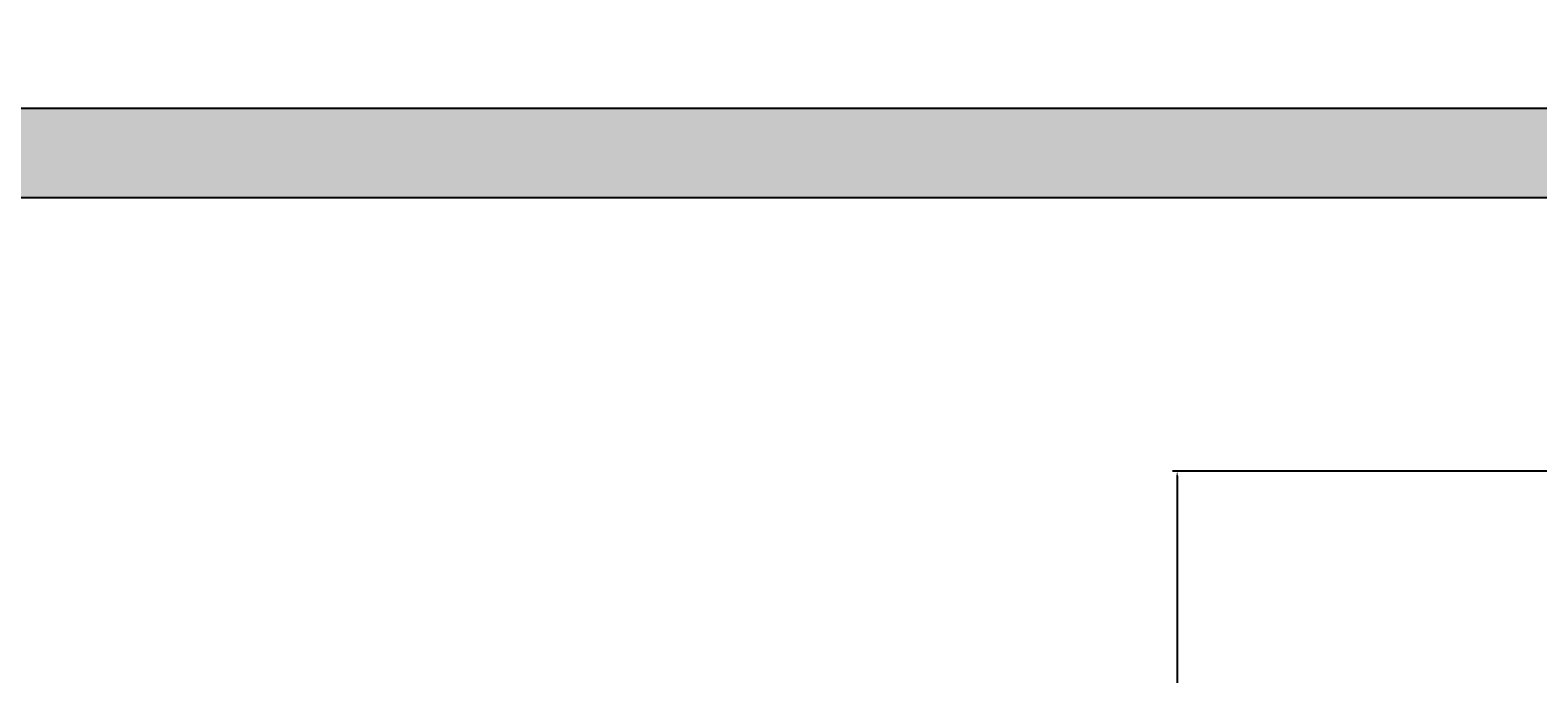
# Model space of a CAD drawing. Units: millimetres. Extents: x -11 to 280, y -4 to 208.
# Tile 20 of 55: x 91 to 150, y 36 to 61. Entities that reach past the tile are written whole.
import ezdxf

# ---------------------------------------------------------------- set-up
doc = ezdxf.new("R2010")
doc.units = ezdxf.units.MM
doc.layers.add('M-DIMS', color=2, linetype='Continuous', lineweight=18)
doc.layers.add('M-HYDR-RETN', color=7, linetype='Continuous', lineweight=25)
doc.layers.add('M-HYDR-RETN-PATT', color=114, linetype='Continuous', lineweight=13, true_color=0x139b48)
doc.styles.get("Standard").update_dxf_attribs({"font": 'arial.ttf'})
doc.dimstyles.get("Standard").update_dxf_attribs({"dimtxt": 0.18, "dimasz": 0.18, "dimexe": 0.18, "dimexo": 0.0625, "dimgap": 0.09, "dimtad": 0, "dimtih": 1, "dimtoh": 1, "dimdec": 4, "dimzin": 0, "dimdsep": 46, "dimtxsty": 'Standard', "dimcen": 0.09, "dimadec": 0, "dimazin": 0, "dimtfac": 1, "dimtdec": 4, "dimtofl": 0, "dimtmove": 0, "dimatfit": 3, "dimfxl": 1, "dimtolj": 1, "dimtzin": 0, "dimarcsym": 0})

# ---------------------------------------------------------------- blocks, each defined once
blk = doc.blocks.new('*D4')
at = {"layer": 'Defpoints', "color": 0, "transparency": 16777216}
for p in [(4.763, 84.426), (266.035, 51.733), (266.035, -3.415)]:
    blk.add_point(p, dxfattribs=at)
at = {"layer": 'M-DIMS', "color": 0, "lineweight": -2, "transparency": 16777216}
for p, q in [((4.763, 84.364), (4.763, -3.595)), ((266.035, 51.67), (266.035, -3.595)), ((4.943, -3.415), (134.934, -3.415)), ((265.855, -3.415), (135.864, -3.415))]:
    blk.add_line(p, q, dxfattribs=at)
at = {"layer": 'M-DIMS', "color": 0, "transparency": 16777216}
for points in [[(4.943, -3.385), (4.943, -3.445), (4.763, -3.415)], [(265.855, -3.385), (265.855, -3.445), (266.035, -3.415)]]:
    blk.add_solid(points, dxfattribs=at)
at = {"layer": 'M-DIMS', "color": 0, "transparency": 16777216, "insert": (135.399, -3.415), "char_height": 0.18, "attachment_point": 5}
blk.add_mtext('\\A1;261.27', dxfattribs=at)
blk = doc.blocks.new('*D5')
at = {"layer": 'Defpoints', "color": 0, "transparency": 16777216}
for p in [(24.759, 192.645), (-10.087, 11.435), (261.686, 11.435)]:
    blk.add_point(p, dxfattribs=at)
at = {"layer": 'M-DIMS', "color": 0, "lineweight": -2, "transparency": 16777216}
for p, q in [((24.696, 192.645), (-10.267, 192.645)), ((-10.087, 192.465), (-10.087, 102.222)), ((-10.087, 11.615), (-10.087, 101.858)), ((261.624, 11.435), (-10.267, 11.435))]:
    blk.add_line(p, q, dxfattribs=at)
at = {"layer": 'M-DIMS', "color": 0, "transparency": 16777216}
for points in [[(-10.117, 192.465), (-10.057, 192.465), (-10.087, 192.645)], [(-10.117, 11.615), (-10.057, 11.615), (-10.087, 11.435)]]:
    blk.add_solid(points, dxfattribs=at)
at = {"layer": 'M-DIMS', "color": 0, "transparency": 16777216, "insert": (-10.087, 102.04), "char_height": 0.18, "attachment_point": 5}
blk.add_mtext('\\A1;181.2', dxfattribs=at)
blk = doc.blocks.new('*D21')
at = {"layer": 'Defpoints', "color": 0, "transparency": 16777216}
for p in [(136.172, 43.599), (151.022, 43.599), (151.022, 22.846)]:
    blk.add_point(p, dxfattribs=at)
at = {"layer": 'M-DIMS', "color": 0, "lineweight": -2, "transparency": 16777216}
for p, q in [((150.959, 43.599), (135.992, 43.599)), ((136.172, 43.419), (136.172, 33.405)), ((136.172, 23.026), (136.172, 33.041)), ((150.959, 22.846), (135.992, 22.846))]:
    blk.add_line(p, q, dxfattribs=at)
at = {"layer": 'M-DIMS', "color": 0, "transparency": 16777216}
for points in [[(136.142, 43.419), (136.202, 43.419), (136.172, 43.599)], [(136.142, 23.026), (136.202, 23.026), (136.172, 22.846)]]:
    blk.add_solid(points, dxfattribs=at)
at = {"layer": 'M-DIMS', "color": 0, "transparency": 16777216, "insert": (136.172, 33.223), "char_height": 0.18, "attachment_point": 5}
blk.add_mtext('\\A1;20.753', dxfattribs=at)

msp = doc.modelspace()

# ---------------------------------------------------------------- hatches: boundary and pattern name
at = {"layer": 'M-HYDR-RETN-PATT'}
h = msp.add_hatch(color=256, dxfattribs=at)
h.set_gradient(color1=(19, 155, 72), color2=(19, 155, 72), tint=1)
h.paths.add_polyline_path([(17.9701, 159.0814), (29.2015, 159.0814), (29.2015, 162.5814), (14.4701, 162.5814), (14.4701, 98.0213), (17.9701, 98.0213)])
h.paths.add_polyline_path([(17.9701, 84.4261), (14.4701, 84.4261), (14.4701, 54.3099), (156.2446, 54.3099), (156.2446, 57.8099), (17.9701, 57.8099)])
h.paths.add_polyline_path([(120.5137, 74.3991), (17.9701, 74.3991), (17.9701, 70.8991), (120.5137, 70.8991)], flags=17)
h.paths.add_polyline_path([(184.7092, 75.04, 0.4142136), (179.7092, 80.04), (156.2446, 80.04), (156.2446, 57.8099), (156.2446, 54.3099), (156.2446, 43.5991), (159.7446, 43.5991), (159.7446, 57.8099), (159.7446, 76.54), (176.2092, 76.54, -0.4142136), (181.2092, 71.54), (181.2092, 57.8099), (159.7446, 57.8099), (159.7446, 54.3099), (184.7092, 54.3099)])

# ---------------------------------------------------------------- linework, layer by layer
at = {"layer": 'M-HYDR-RETN'}
for points in [[(14.4701, 84.4261), (14.4701, 54.3099), (156.2446, 54.3099)], [(17.9701, 84.4261), (17.9701, 57.8099), (156.2446, 57.8099)]]:
    msp.add_lwpolyline(points, dxfattribs=at)

# ---------------------------------------------------------------- dimensions: what is measured, and where the dimension line sits
at = {"layer": 'M-DIMS'}
for base, p1, p2, override, picture, middle in [((-10.0865, 11.4346), (24.7588, 192.645), (261.6863, 11.4346), {"dimdec": 1, "dimlfac": 1, "dimrnd": 0, "dimzin": 0, "dimdsep": 46, "dimlunit": 2}, '*D5', (-10.0865, 102.0398)), ((136.1717, 43.5991), (151.0217, 22.846), (151.0217, 43.5991), {"dimdec": 3, "dimlfac": 1, "dimrnd": 0, "dimzin": 0, "dimdsep": 46, "dimlunit": 2}, '*D21', (136.1717, 33.2226))]:
    dim = msp.add_linear_dim(base=base, p1=p1, p2=p2, angle=90, dimstyle='Standard', override=override, dxfattribs=at)
    dim.commit()
    dim.dimension.update_dxf_attribs({"geometry": picture, "text_midpoint": middle})
dim = msp.add_linear_dim(base=(266.0352, -3.4154), p1=(4.7635, 84.4261), p2=(266.0352, 51.7328), dimstyle='Standard', override={"dimdec": 2, "dimlfac": 1, "dimrnd": 0, "dimzin": 0, "dimdsep": 46, "dimlunit": 2}, dxfattribs=at)
dim.commit()
dim.dimension.update_dxf_attribs({"geometry": '*D4', "text_midpoint": (135.3993, -3.4154)})

doc.saveas('drawing.dxf')
